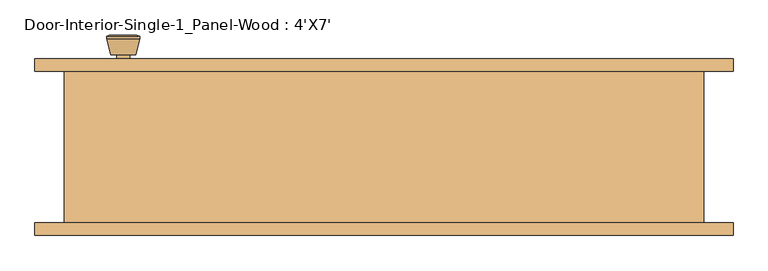
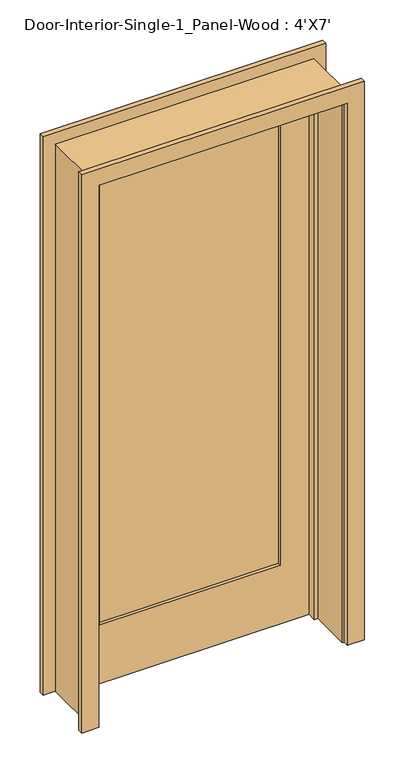
"""IFC4 building model written with IfcOpenShell, lengths in millimetres: door geometry, Door-Interior-Single-1_Panel-Wood : 4'X7'."""

from ifc_helpers import new_model, si_unit, point, frame, frame_2d, origin, place, context, project, spatial, polyline, circle_curve, trimmed, segment, composite_curve, outline, extrude, faceted_brep, source, transform, mapped, element, save
from ifc_brep_helpers import plane_surface, cylinder_surface, revolved_surface, advanced_brep


def door_interior_single_1_panel_wood_4_x7_3b97b8e7(model_context):
    return source(origin(), model_context, "Body", "SolidModel", [
        advanced_brep(
        [(-393.7, 70.2, 914.4), (-383.7, 70.2, 914.4), (-403.7, 70.2, 914.4), (-373.2241324, 21.2, 914.4), (-393.7, 21.2, 914.4), (-414.1758676, 21.2, 914.4), (-368.7, 23.0278681, 914.4), (-418.7, 23.0278681, 914.4), (-368.7, 26.4915463, 914.4), (-418.7, 26.4915463, 914.4), (-375.063764, 51.2, 914.4), (-412.336236, 51.2, 914.4), (-383.7, 51.2, 914.4), (-403.7, 51.2, 914.4)],
        [
            (0, 1),
            (1, 2, circle_curve(frame((-393.7, 70.2, 914.4), z_axis=(0.0, 1.0, 0.0), x_axis=(-1.0, 0.0, 0.0)), 10.0)),
            (2, 0),
            (2, 1, circle_curve(frame((-393.7, 70.2, 914.4), z_axis=(0.0, 1.0, 0.0), x_axis=(-1.0, 0.0, 0.0)), 10.0)),
            (3, 4),
            (4, 5),
            (5, 3, circle_curve(frame((-393.7, 21.2, 914.4), z_axis=(0.0, -1.0, 0.0), x_axis=(-1.0, 0.0, 0.0)), 20.4758676)),
            (3, 5, circle_curve(frame((-393.7, 21.2, 914.4), z_axis=(0.0, -1.0, 0.0), x_axis=(-1.0, 0.0, 0.0)), 20.4758676)),
            (6, 3),
            (5, 7),
            (7, 6, circle_curve(frame((-393.7, 23.0278681, 914.4), z_axis=(0.0, -1.0, 0.0), x_axis=(-1.0, 0.0, 0.0)), 25.0)),
            (6, 7, circle_curve(frame((-393.7, 23.0278681, 914.4), z_axis=(0.0, -1.0, 0.0), x_axis=(-1.0, 0.0, 0.0)), 25.0)),
            (8, 6),
            (7, 9),
            (9, 8, circle_curve(frame((-393.7, 26.4915463, 914.4), z_axis=(0.0, -1.0, 0.0), x_axis=(-1.0, 0.0, 0.0)), 25.0)),
            (8, 9, circle_curve(frame((-393.7, 26.4915463, 914.4), z_axis=(0.0, -1.0, 0.0), x_axis=(-1.0, 0.0, 0.0)), 25.0)),
            (10, 8),
            (9, 11),
            (11, 10, circle_curve(frame((-393.7, 51.2, 914.4), z_axis=(0.0, -1.0, 0.0), x_axis=(-1.0, 0.0, 0.0)), 18.636236)),
            (10, 11, circle_curve(frame((-393.7, 51.2, 914.4), z_axis=(0.0, -1.0, 0.0), x_axis=(-1.0, 0.0, 0.0)), 18.636236)),
            (12, 10),
            (11, 13),
            (13, 12, circle_curve(frame((-393.7, 51.2, 914.4), z_axis=(0.0, -1.0, 0.0), x_axis=(-1.0, 0.0, 0.0)), 10.0)),
            (12, 13, circle_curve(frame((-393.7, 51.2, 914.4), z_axis=(0.0, -1.0, 0.0), x_axis=(-1.0, 0.0, 0.0)), 10.0)),
            (1, 12),
            (13, 2),
        ],
        [
            plane_surface(frame((-393.7, 70.2, 914.4), z_axis=(0.0, 1.0, 0.0), x_axis=(-1.0, 0.0, 0.0))),
            plane_surface(frame((-393.7, 21.2, 914.4), z_axis=(0.0, -1.0, 0.0), x_axis=(-1.0, 0.0, 0.0))),
            revolved_surface(polyline([(-414.1758676, 21.2, 914.4), (-418.7, 23.0278681, 914.4)]), (-393.7, 70.2, 914.4), (0.0, 1.0, 0.0)),
            cylinder_surface(frame((-393.7, 70.2, 914.4), z_axis=(0.0, 1.0, 0.0), x_axis=(-1.0, 0.0, 0.0)), 25.0),
            revolved_surface(polyline([(-418.7, 26.4915463, 914.4), (-412.336236, 51.2, 914.4)]), (-393.7, 70.2, 914.4), (0.0, 1.0, 0.0)),
            plane_surface(frame((-393.7, 51.2, 914.4), z_axis=(0.0, 1.0, 0.0), x_axis=(-1.0, 0.0, 0.0))),
            cylinder_surface(frame((-393.7, 70.2, 914.4), z_axis=(0.0, 1.0, 0.0), x_axis=(-1.0, 0.0, 0.0)), 10.0),
        ],
        [
            (0, [[1, 2, 3]]),
            (0, [[-3, 4, -1]]),
            (1, [[5, 6, 7]]),
            (1, [[-6, -5, 8]]),
            (2, [[9, -7, 10, 11]]),
            (2, [[-10, -8, -9, 12]]),
            (3, [[13, -11, 14, 15]]),
            (3, [[-14, -12, -13, 16]]),
            (4, [[17, -15, 18, 19]]),
            (4, [[-18, -16, -17, 20]]),
            (5, [[21, -19, 22, 23]]),
            (5, [[-22, -20, -21, 24]]),
            (6, [[25, -23, 26, -2]]),
            (6, [[-26, -24, -25, -4]]),
        ],
    ),
        extrude(outline(composite_curve([segment(trimmed(circle_curve(frame_2d((914.4, -393.7)), 30.0), [point((914.4, -423.7))], [point((914.4, -363.7))], False, "CARTESIAN"), True, "CONTINUOUS"), segment(trimmed(circle_curve(frame_2d((914.4, -393.7)), 30.0), [point((914.4, -363.7))], [point((914.4, -423.7))], False, "CARTESIAN"), True, "CONTINUOUS")], self_intersect=False)), frame((0.0, 70.2, 0.0), z_axis=(0.0, 1.0, 0.0), x_axis=(0.0, 0.0, 1.0)), (0.0, 0.0, 1.0), 6.0),
        advanced_brep(
        [(-393.7, 117.125, 914.4), (-403.7, 117.125, 914.4), (-383.7, 117.125, 914.4), (-373.2241324, 166.125, 914.4), (-414.1758676, 166.125, 914.4), (-393.7, 166.125, 914.4), (-368.7, 164.2971319, 914.4), (-418.7, 164.2971319, 914.4), (-368.7, 160.8334537, 914.4), (-418.7, 160.8334537, 914.4), (-375.063764, 136.125, 914.4), (-412.336236, 136.125, 914.4), (-383.7, 136.125, 914.4), (-403.7, 136.125, 914.4)],
        [
            (0, 1),
            (1, 2, circle_curve(frame((-393.7, 117.125, 914.4), z_axis=(0.0, -1.0, 0.0), x_axis=(-1.0, 0.0, 0.0)), 10.0)),
            (2, 0),
            (2, 1, circle_curve(frame((-393.7, 117.125, 914.4), z_axis=(0.0, -1.0, 0.0), x_axis=(-1.0, 0.0, 0.0)), 10.0)),
            (3, 4, circle_curve(frame((-393.7, 166.125, 914.4), z_axis=(0.0, 1.0, 0.0), x_axis=(-1.0, 0.0, 0.0)), 20.4758676)),
            (4, 5),
            (5, 3),
            (4, 3, circle_curve(frame((-393.7, 166.125, 914.4), z_axis=(0.0, 1.0, 0.0), x_axis=(-1.0, 0.0, 0.0)), 20.4758676)),
            (6, 7, circle_curve(frame((-393.7, 164.2971319, 914.4), z_axis=(0.0, 1.0, 0.0), x_axis=(-1.0, 0.0, 0.0)), 25.0)),
            (7, 4),
            (3, 6),
            (7, 6, circle_curve(frame((-393.7, 164.2971319, 914.4), z_axis=(0.0, 1.0, 0.0), x_axis=(-1.0, 0.0, 0.0)), 25.0)),
            (8, 9, circle_curve(frame((-393.7, 160.8334537, 914.4), z_axis=(0.0, 1.0, 0.0), x_axis=(-1.0, 0.0, 0.0)), 25.0)),
            (9, 7),
            (6, 8),
            (9, 8, circle_curve(frame((-393.7, 160.8334537, 914.4), z_axis=(0.0, 1.0, 0.0), x_axis=(-1.0, 0.0, 0.0)), 25.0)),
            (10, 11, circle_curve(frame((-393.7, 136.125, 914.4), z_axis=(0.0, 1.0, 0.0), x_axis=(-1.0, 0.0, 0.0)), 18.636236)),
            (11, 9),
            (8, 10),
            (11, 10, circle_curve(frame((-393.7, 136.125, 914.4), z_axis=(0.0, 1.0, 0.0), x_axis=(-1.0, 0.0, 0.0)), 18.636236)),
            (12, 13, circle_curve(frame((-393.7, 136.125, 914.4), z_axis=(0.0, 1.0, 0.0), x_axis=(-1.0, 0.0, 0.0)), 10.0)),
            (13, 11),
            (10, 12),
            (13, 12, circle_curve(frame((-393.7, 136.125, 914.4), z_axis=(0.0, 1.0, 0.0), x_axis=(-1.0, 0.0, 0.0)), 10.0)),
            (1, 13),
            (12, 2),
        ],
        [
            plane_surface(frame((-393.7, 117.125, 914.4), z_axis=(0.0, -1.0, 0.0), x_axis=(-1.0, 0.0, 0.0))),
            plane_surface(frame((-393.7, 166.125, 914.4), z_axis=(0.0, 1.0, 0.0), x_axis=(-1.0, 0.0, 0.0))),
            revolved_surface(polyline([(-414.1758676, 166.125, 914.4), (-418.7, 164.2971319, 914.4)]), (-393.7, 117.125, 914.4), (0.0, -1.0, 0.0)),
            cylinder_surface(frame((-393.7, 117.125, 914.4), z_axis=(0.0, -1.0, 0.0), x_axis=(-1.0, 0.0, 0.0)), 25.0),
            revolved_surface(polyline([(-418.7, 160.8334537, 914.4), (-412.336236, 136.125, 914.4)]), (-393.7, 117.125, 914.4), (0.0, -1.0, 0.0)),
            plane_surface(frame((-393.7, 136.125, 914.4), z_axis=(0.0, -1.0, 0.0), x_axis=(-1.0, 0.0, 0.0))),
            cylinder_surface(frame((-393.7, 117.125, 914.4), z_axis=(0.0, -1.0, 0.0), x_axis=(-1.0, 0.0, 0.0)), 10.0),
        ],
        [
            (0, [[1, 2, 3]]),
            (0, [[-3, 4, -1]]),
            (1, [[5, 6, 7]]),
            (1, [[8, -7, -6]]),
            (2, [[9, 10, -5, 11]]),
            (2, [[12, -11, -8, -10]]),
            (3, [[13, 14, -9, 15]]),
            (3, [[16, -15, -12, -14]]),
            (4, [[17, 18, -13, 19]]),
            (4, [[20, -19, -16, -18]]),
            (5, [[21, 22, -17, 23]]),
            (5, [[24, -23, -20, -22]]),
            (6, [[-2, 25, -21, 26]]),
            (6, [[-4, -26, -24, -25]]),
        ],
    ),
        extrude(outline(composite_curve([segment(trimmed(circle_curve(frame_2d((914.4, -393.7)), 30.0), [point((914.4, -423.7))], [point((914.4, -363.7))], False, "CARTESIAN"), True, "CONTINUOUS"), segment(trimmed(circle_curve(frame_2d((914.4, -393.7)), 30.0), [point((914.4, -363.7))], [point((914.4, -423.7))], False, "CARTESIAN"), True, "CONTINUOUS")], self_intersect=False)), frame((0.0, 111.125, 0.0), z_axis=(0.0, 1.0, 0.0), x_axis=(0.0, 0.0, 1.0)), (0.0, 0.0, 1.0), 6.0),
        faceted_brep([(482.6, 111.125, 0.0), (482.6, -117.475, 0.0), (457.2, -117.475, 0.0), (457.2, 41.275, 0.0), (444.5, 41.275, 0.0), (444.5, 76.2, 0.0), (457.2, 76.2, 0.0), (457.2, 111.125, 0.0), (482.6, 111.125, 2159.0), (482.6, -117.475, 2159.0), (-482.6, -117.475, 2159.0), (-482.6, -117.475, 0.0), (-457.2, -117.475, 0.0), (-457.2, -117.475, 2133.6), (457.2, -117.475, 2133.6), (457.2, 41.275, 2133.6), (-457.2, 41.275, 2133.6), (-457.2, 41.275, 0.0), (-444.5, 41.275, 0.0), (-444.5, 41.275, 2120.9), (444.5, 41.275, 2120.9), (444.5, 76.2, 2120.9), (-444.5, 76.2, 2120.9), (-444.5, 76.2, 0.0), (-457.2, 76.2, 0.0), (-457.2, 76.2, 2133.6), (457.2, 76.2, 2133.6), (457.2, 111.125, 2133.6), (-457.2, 111.125, 2133.6), (-457.2, 111.125, 0.0), (-482.6, 111.125, 0.0), (-482.6, 111.125, 2159.0)], [[[0, 1, 2, 3, 4, 5, 6, 7]], [[1, 0, 8, 9]], [[2, 1, 9, 10, 11, 12, 13, 14]], [[3, 2, 14, 15]], [[4, 3, 15, 16, 17, 18, 19, 20]], [[5, 4, 20, 21]], [[6, 5, 21, 22, 23, 24, 25, 26]], [[7, 6, 26, 27]], [[0, 7, 27, 28, 29, 30, 31, 8]], [[9, 8, 31, 10]], [[15, 14, 13, 16]], [[21, 20, 19, 22]], [[27, 26, 25, 28]], [[30, 29, 24, 23, 18, 17, 12, 11]], [[10, 31, 30, 11]], [[16, 13, 12, 17]], [[22, 19, 18, 23]], [[28, 25, 24, 29]]]),
        extrude(outline(polyline([(2133.6, -457.2), (0.0, -457.2), (0.0, 457.2), (2133.6, 457.2), (2133.6, -457.2)]), holes=[polyline([(2014.5375, -336.55), (2014.5375, 336.55), (231.775, 336.55), (231.775, -336.55), (2014.5375, -336.55)])]), frame((0.0, 76.2, 0.0), z_axis=(0.0, 1.0, 0.0), x_axis=(0.0, 0.0, 1.0)), (0.0, 0.0, 1.0), 34.925),
        extrude(outline(polyline([(336.55, 87.8416667), (-336.55, 87.8416667), (-336.55, 99.4833333), (336.55, 99.4833333), (336.55, 87.8416667)])), frame((0.0, 0.0, 231.775), z_axis=(0.0, 0.0, 1.0), x_axis=(1.0, 0.0, 0.0)), (0.0, 0.0, 1.0), 1782.7625),
        extrude(outline(polyline([(0.0, 463.55), (0.0, 527.05), (2203.45, 527.05), (2203.45, -527.05), (0.0, -527.05), (0.0, -463.55), (2139.95, -463.55), (2139.95, 463.55), (0.0, 463.55)])), frame((0.0, 111.125, 0.0), z_axis=(0.0, 1.0, 0.0), x_axis=(0.0, 0.0, 1.0)), (0.0, 0.0, 1.0), 19.05),
        extrude(outline(polyline([(0.0, 463.55), (0.0, 527.05), (2203.45, 527.05), (2203.45, -527.05), (0.0, -527.05), (0.0, -463.55), (2139.95, -463.55), (2139.95, 463.55), (0.0, 463.55)])), frame((0.0, -136.525, 0.0), z_axis=(0.0, 1.0, 0.0), x_axis=(0.0, 0.0, 1.0)), (0.0, 0.0, 1.0), 19.05),
    ])


if __name__ == "__main__":
    model = new_model("IFC4")
    model_context = context("Model", 3, world=origin())
    ifc_project = project(units=[si_unit("LENGTHUNIT", "METRE", prefix="MILLI")], contexts=[model_context])
    site = spatial("IfcSite", under=ifc_project)
    building = spatial("IfcBuilding", under=site)
    placement = place(None, origin())
    door_interior_single_1_panel_wood_4_x7_shape = door_interior_single_1_panel_wood_4_x7_3b97b8e7(model_context)
    element("IfcDoor", 1, ObjectType="Door-Interior-Single-1_Panel-Wood : 4'X7'", at=placement, inside=building, context=model_context, shape_type="MappedRepresentation", body=[
        mapped(door_interior_single_1_panel_wood_4_x7_shape, transform((0.0, 0.0, 0.0), x_axis=(1.0, 0.0, 0.0), y_axis=(0.0, 1.0, 0.0), z_axis=(0.0, 0.0, 1.0))),
    ])
    save(model, "model.ifc")

# Revit data of these elements
# Type "Door-Interior-Single-1_Panel-Wood : 4'X7'"
#   Type Mark = "9"
#   Assembly Code = "C1020300"
#   Analytic Construction = "Wooden"
#   Top Rail = 0' - 4 11/16"
#   Thickness = 0' - 1 3/8"
#   Thermal Resistance (R) = 2.5876 (h·ft²·°F)/BTU
#   Swing Angle [instance default] = 90.00°
#   Stiles = 0' - 4 3/4"
#   Rough Width = 3' - 2"
#   Rough Height = 7' - 1"
#   Height = 7' - 0"
#   Width = 3' - 0"
#   Heat Transfer Coefficient (U) = 0.3865 BTU/(h·ft²·°F)
#   Bottom Rail = 0' - 9 1/8"
#   Trim Material = Cherry
#   Panel Material = Cherry
#   Frame Material = Cherry
#   Door Handle Material = Aluminum
#   Visual Light Transmittance = 0
#   Solar Heat Gain Coefficient = 0
#   Wall Closure = (empty or 0)
#   Function = (empty or 0)
# Element 1 (IfcDoor, "Door-Interior-Single-1_Panel-Wood : 4'X7'")
#   Materials on its faces: "Cherry", "Aluminum"
# Materials
#   "Cherry": class "Wood", colour RGB 226 177 128, transparency 0, Description = "Prunus Serotina", Cost = 0
#   "Aluminum": class "Metal", colour RGB 247 247 247, transparency 0, Description = "Aluminum 6061", Cost = 0
